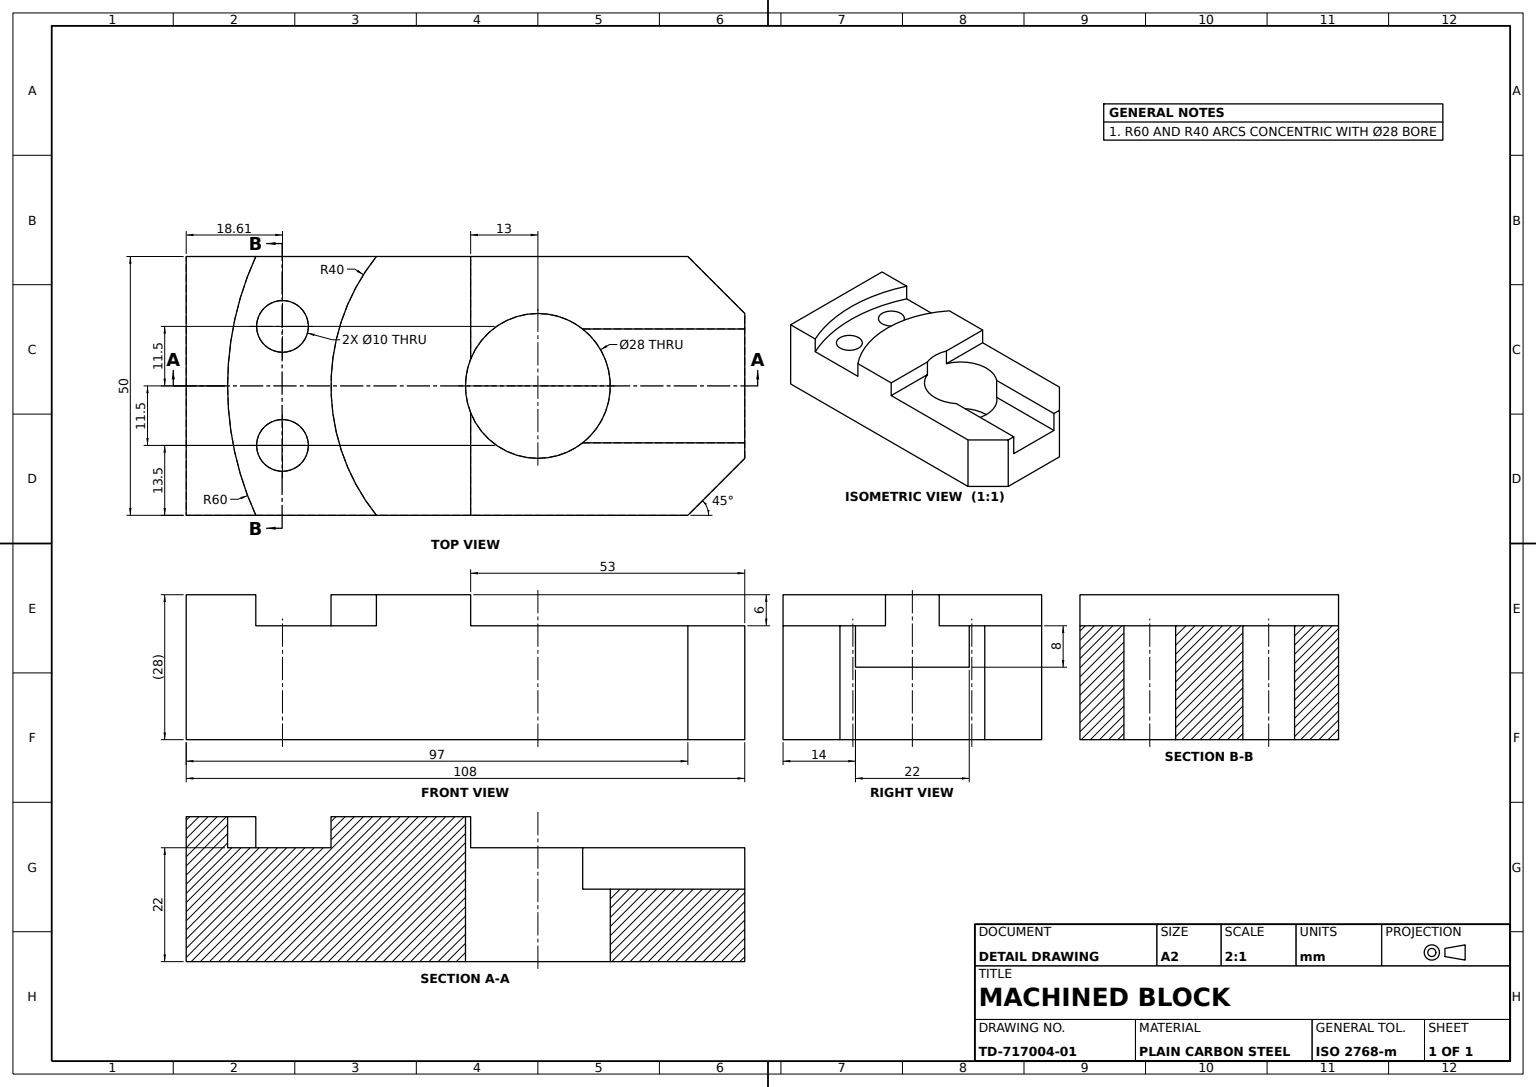
SolidWorks part; units mm, degrees
material "Plain Carbon Steel"
ref_plane "Front Plane" through (0, 0, 0) normal (0, 0, 1) x (1, 0, 0)
ref_plane "Top Plane" through (0, 0, 0) normal (0, 1, 0) x (1, 0, 0)
ref_plane "Right Plane" through (0, 0, 0) normal (1, 0, 0) x (0, 0, -1)
sketch "Base Block Profile" plane through (0, 0, 0) normal (0, 1, 0) x (1, 0, 0)
  line L1 (-54, 25) -> (43, 25)
  line L2 (-54, 25) -> (-54, -25)
  line L3 (-54, -25) -> (43, -25)
  line L5 (-54, 25) -> (54, -25) construction
  line L6 (-54, -25) -> (54, 25) construction
  line L8 (43, -25) -> (54, -25)
  line L9 (54, -25) -> (54, 25)
  line L10 (54, 25) -> (43, 25)
  point P0 (0, 0)
  dimension "D1" = 50
  dimension "D2" = 108
  dimension "D3" = 97
extrude "Base Block 108x50x28" add sketch "Base Block Profile" along normal blind 28
sketch "Jaw Slot Profile" plane through (54, 0, 0) normal (1, 0, 0) x (0, 0, -1)
  line L0 (-25, 28) -> (25, 28) construction
  line L1 (-11, 28) -> (11, 28)
  line L2 (-11, 28) -> (-11, 22)
  line L3 (-11, 22) -> (11, 22)
  line L4 (11, 28) -> (11, 22)
  dimension "D1" = 11
  dimension "D2" = 22
  dimension "D3" = 6
extrude "Jaw Slot Cut" cut sketch "Jaw Slot Profile" against normal blind 40
sketch "Bore Ø28 Profile" plane through (0, 28, 0) normal (0, 1, 0) x (1, 0, 0)
  line L0 (14, 11) -> (14, -11) construction
  circle A0 centre (14, 0) radius 14
  dimension "D1" = 28
extrude "Bore Ø28" cut sketch "Bore Ø28 Profile" against normal through all
sketch "Through Slot Profile" plane through (54, 0, 0) normal (1, 0, 0) x (0, 0, -1)
  line L1 (-25, 28) -> (-11, 28)
  line L2 (-25, 28) -> (-25, 22)
  line L3 (-25, 22) -> (-11, 22)
  line L9 (-11, 28) -> (25, 28)
  line L10 (25, 28) -> (25, 22)
  line L11 (25, 28) -> (25, 0) construction
  line L12 (25, 22) -> (-11, 22)
extrude "Through Slot Cut" cut sketch "Through Slot Profile" against normal blind 53
sketch "Side Groove Profile" plane through (54, 0, 0) normal (1, 0, 0) x (0, 0, -1)
  line L0 (-25, 22) -> (25, 22) construction
  line L1 (-11, 22) -> (11, 22)
  line L2 (-11, 22) -> (-11, 14)
  line L3 (-11, 14) -> (11, 14)
  line L4 (11, 22) -> (11, 14)
  line L5 (-25, 0) -> (25, 0) construction
  point P8 (0, 0)
  dimension "D1" = 8
  dimension "D2" = 11
  dimension "D3" = 22
extrude "Side Groove Cut" cut sketch "Side Groove Profile" against normal blind 40
chamfer "End Chamfer 11x45°" distance 11 angle 45 2 edges at (54, 11, -25) (54, 11, 25)
sketch "Arc Recess Profile" plane through (0, 28, 0) normal (0, 1, 0) x (1, 0, 0)
  line L0 (-54, -25) -> (1, -25) construction
  line L1 (1, 25) -> (-54, 25) construction
  line L2 (-40.5436, -25) -> (-17.225, -25)
  line L3 (-17.225, 25) -> (-40.5436, 25)
  line L4 (1, -5.1962) -> (1, -25) construction
  arc A8 (-29.3013, 25) -> (-29.3013, -25) centre (14, 0) ccw construction
  arc A9 (-40.5436, 25) -> (-40.5436, -25) centre (14, 0) ccw
  arc A10 (-17.225, 25) -> (-17.225, -25) centre (14, 0) ccw
  dimension "D1" = 100
  dimension "D2" = 120
  dimension "D3" = 80
  dimension "D4" = 13
extrude "Arc Recess 6 Deep" cut sketch "Arc Recess Profile" against normal blind 6
sketch "Arc Pocket and Holes Profile" plane through (0, 28, 0) normal (0, 1, 0) x (1, 0, 0)
  line L0 (0, 0) -> (-70.2009, 0) construction
  line L1 (0, 0) -> (-67.4216, 21.9066) construction
  line L2 (0, 0) -> (-69.0739, -22.4435) construction
  line L3 (1, -5.1962) -> (1, -25) construction
  arc A1 (1, 5.1962) -> (1, -5.1962) centre (14, 0) ccw construction
  arc A5 (1, 5.1962) -> (0, 0) centre (14, 0) ccw
  circle A8 centre (13.2748, 0) radius 50 construction
  circle A9 centre (-35.3854, 11.4974) radius 5
  circle A10 centre (-35.3854, -11.4974) radius 5
  dimension "D3" = 100
  dimension "D4" = 10
  dimension "D5" = 10
  dimension "D1" = 18
  dimension "D2" = 18
  dimension "D6" = 12.2748
extrude "Arc Pocket and Holes Cut" cut sketch "Arc Pocket and Holes Profile" against normal through all contours A9 | A10
